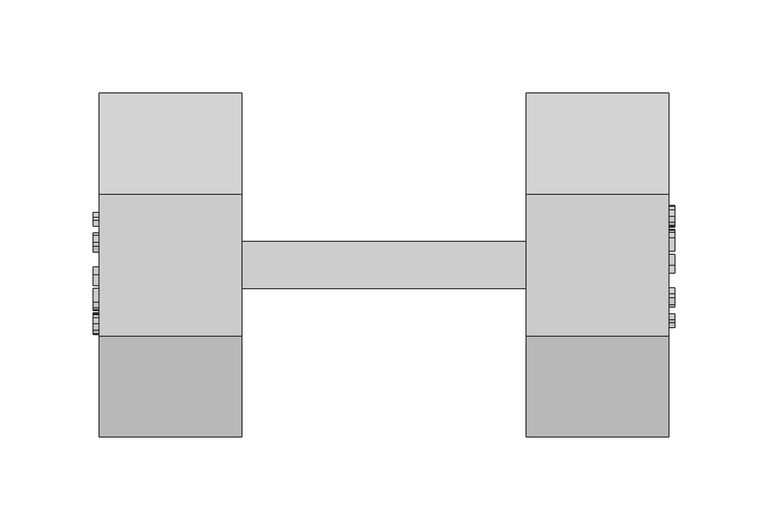
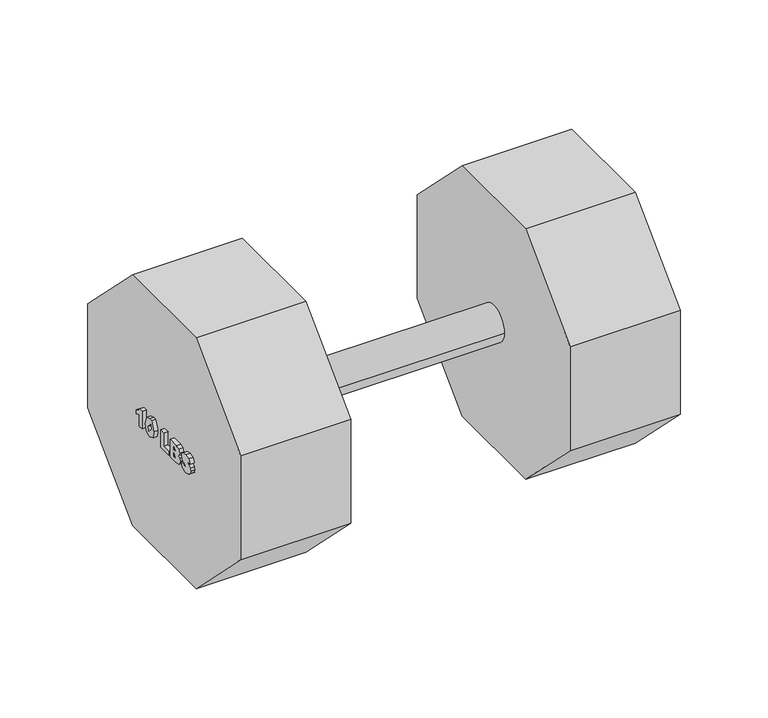
"""IFC4 building model written with IfcOpenShell, lengths in millimetres: proxy geometry."""

from ifc_helpers import new_model, si_unit, point, frame, frame_2d, origin, place, context, project, spatial, polyline, circle_curve, trimmed, segment, composite_curve, outline, extrude, source, transform, mapped, element, save


def generic_models_59bf1475(model_context):
    return source(origin(), model_context, "Body", "SweptSolid", [
        extrude(outline(polyline([(91.9815367, 53.8815367), (38.1, 0.0), (-38.1, 0.0), (-91.9815367, 53.8815367), (-91.9815367, 130.0815367), (-38.1, 183.9630735), (38.1, 183.9630735), (91.9815367, 130.0815367), (91.9815367, 53.8815367)])), frame((-76.2, 0.0, 0.0), z_axis=(1.0, 0.0, 0.0), x_axis=(0.0, 1.0, 0.0)), (0.0, 0.0, 1.0), 76.2),
        extrude(outline(composite_curve([segment(trimmed(circle_curve(frame_2d((0.0, 91.9815367)), 12.7), [point((12.7, 91.9815367))], [point((-12.7, 91.9815367))], False, "CARTESIAN"), True, "CONTINUOUS"), segment(trimmed(circle_curve(frame_2d((0.0, 91.9815367)), 12.7), [point((-12.7, 91.9815367))], [point((12.7, 91.9815367))], False, "CARTESIAN"), True, "CONTINUOUS")], self_intersect=False)), frame((0.0, 0.0, 0.0), z_axis=(1.0, 0.0, 0.0), x_axis=(0.0, 1.0, 0.0)), (0.0, 0.0, 1.0), 152.4),
        extrude(outline(polyline([(91.9815367, 53.8815367), (38.1, 0.0), (-38.1, 0.0), (-91.9815367, 53.8815367), (-91.9815367, 130.0815367), (-38.1, 183.9630735), (38.1, 183.9630735), (91.9815367, 130.0815367), (91.9815367, 53.8815367)])), frame((152.4, 0.0, 0.0), z_axis=(1.0, 0.0, 0.0), x_axis=(0.0, 1.0, 0.0)), (0.0, 0.0, 1.0), 76.2),
        extrude(outline(polyline([(20.9176471, 95.3120931), (23.7696998, 95.3120931), (25.3338542, 93.4016458), (28.1392157, 92.0748382), (28.1392157, 89.0866029), (26.0925858, 89.8920257), (24.4039216, 90.9931592), (24.4039216, 82.3630735), (20.9176471, 82.3630735), (20.9176471, 95.3120931)])), frame((-79.375, 0.0, 0.0), z_axis=(1.0, 0.0, 0.0), x_axis=(0.0, 1.0, 0.0)), (0.0, 0.0, 1.0), 3.175),
        extrude(outline(polyline([(17.1823529, 88.7636556), (16.9313879, 86.0614037), (16.2290748, 84.1334472), (14.6337929, 82.6276568), (12.0852328, 82.1140538), (8.1223192, 83.7248994), (6.972549, 88.8103467), (9.921875, 94.9949822), (11.9918505, 95.3120931), (15.9002911, 93.8588302), (17.1823529, 88.7636556)]), holes=[polyline([(13.6960784, 88.7247462), (10.8712623, 91.9678375), (10.4588235, 88.6313639), (13.2836397, 85.4758186), (13.6960784, 88.7247462)])]), frame((-79.375, 0.0, 0.0), z_axis=(1.0, 0.0, 0.0), x_axis=(0.0, 1.0, 0.0)), (0.0, 0.0, 1.0), 3.175),
        extrude(outline(polyline([(-0.9960784, 95.0630735), (-0.9960784, 82.3630735), (-10.9568627, 82.3630735), (-10.9568627, 85.3513087), (-4.9803922, 85.3513087), (-4.9803922, 95.0630735), (-0.9960784, 95.0630735)])), frame((-79.375, 0.0, 0.0), z_axis=(1.0, 0.0, 0.0), x_axis=(0.0, 1.0, 0.0)), (0.0, 0.0, 1.0), 3.175),
        extrude(outline(polyline([(-12.7, 95.0630735), (-12.7, 82.3630735), (-19.4546569, 82.3630735), (-22.6919118, 82.9506041), (-23.9467371, 84.1918112), (-24.4039216, 85.958294), (-23.7619179, 87.9660146), (-21.7619792, 89.0904938), (-23.1782782, 89.9426078), (-23.9058824, 91.8841825), (-22.9175858, 94.1487046), (-20.0849877, 95.0630735), (-12.7, 95.0630735)]), holes=[polyline([(-16.6843137, 85.3513087), (-16.6843137, 87.5924852), (-18.6258885, 85.3513087), (-16.6843137, 85.3513087)]), polyline([(-16.6843137, 90.0826813), (-16.6843137, 92.0748382), (-18.3379596, 90.0826813), (-16.6843137, 90.0826813)])]), frame((-79.375, 0.0, 0.0), z_axis=(1.0, 0.0, 0.0), x_axis=(0.0, 1.0, 0.0)), (0.0, 0.0, 1.0), 3.175),
        extrude(outline(polyline([(-25.6490196, 86.6041886), (-27.0536458, 83.3824975), (-31.5126532, 82.1140538), (-34.5553615, 82.6548933), (-36.4327359, 84.2443388), (-37.1039216, 86.530261), (-36.6019914, 88.4426537), (-34.9950368, 89.872571), (-32.6215686, 91.3277793), (-36.6058824, 91.5573443), (-35.1098192, 94.4132879), (-31.4581801, 95.3120931), (-28.3843444, 94.8140538), (-26.7054075, 93.4483369), (-26.1470588, 91.6040355), (-27.2481924, 89.1566396), (-30.897886, 87.6002671), (-31.5865809, 84.6042499), (-29.6333333, 86.8454264), (-25.6490196, 86.6041886)])), frame((-79.375, 0.0, 0.0), z_axis=(1.0, 0.0, 0.0), x_axis=(0.0, 1.0, 0.0)), (0.0, 0.0, 1.0), 3.175),
        extrude(outline(polyline([(-26.2557919, 99.036487), (-26.2557919, 86.0874674), (-29.7420665, 86.0874674), (-29.7420665, 94.7175531), (-31.4307307, 93.6164196), (-33.4773606, 92.8109968), (-33.4773606, 95.7992321), (-30.6719991, 97.1260397), (-29.1078446, 99.036487), (-26.2557919, 99.036487)])), frame((228.6, 0.0, 0.0), z_axis=(1.0, 0.0, 0.0), x_axis=(0.0, 1.0, 0.0)), (0.0, 0.0, 1.0), 3.175),
        extrude(outline(polyline([(-22.5204978, 92.4880495), (-21.2384359, 97.5832241), (-17.3299954, 99.036487), (-15.2600199, 98.7193761), (-12.3106939, 92.5347406), (-13.4604641, 87.4492933), (-17.4233777, 85.8384478), (-19.9719378, 86.3520507), (-21.5672196, 87.8578411), (-22.2695328, 89.7857976), (-22.5204978, 92.4880495)]), holes=[polyline([(-19.0342233, 92.4491402), (-18.6217846, 89.2002125), (-15.7969684, 92.3557578), (-16.2094071, 95.6922315), (-19.0342233, 92.4491402)])]), frame((228.6, 0.0, 0.0), z_axis=(1.0, 0.0, 0.0), x_axis=(0.0, 1.0, 0.0)), (0.0, 0.0, 1.0), 3.175),
        extrude(outline(polyline([(-4.3420665, 98.7874674), (-0.3577527, 98.7874674), (-0.3577527, 89.0757027), (5.6187179, 89.0757027), (5.6187179, 86.0874674), (-4.3420665, 86.0874674), (-4.3420665, 98.7874674)])), frame((228.6, 0.0, 0.0), z_axis=(1.0, 0.0, 0.0), x_axis=(0.0, 1.0, 0.0)), (0.0, 0.0, 1.0), 3.175),
        extrude(outline(polyline([(7.3618551, 98.7874674), (14.7468429, 98.7874674), (17.5794409, 97.8730985), (18.5677375, 95.6085764), (17.8401333, 93.6670017), (16.4238343, 92.8148877), (18.423773, 91.6904085), (19.0657767, 89.682688), (18.6085922, 87.9162051), (17.3537669, 86.674998), (14.116512, 86.0874674), (7.3618551, 86.0874674), (7.3618551, 98.7874674)]), holes=[polyline([(11.3461688, 93.8070752), (12.9998147, 93.8070752), (11.3461688, 95.7992321), (11.3461688, 93.8070752)]), polyline([(11.3461688, 89.0757027), (13.2877436, 89.0757027), (11.3461688, 91.3168791), (11.3461688, 89.0757027)])]), frame((228.6, 0.0, 0.0), z_axis=(1.0, 0.0, 0.0), x_axis=(0.0, 1.0, 0.0)), (0.0, 0.0, 1.0), 3.175),
        extrude(outline(polyline([(20.3108747, 90.3285826), (24.2951884, 90.5698203), (26.248436, 88.3286438), (25.5597411, 91.324661), (21.9100475, 92.8810335), (20.8089139, 95.3284294), (21.3672626, 97.1727308), (23.0461995, 98.5384478), (26.1200353, 99.036487), (29.7716744, 98.1376818), (31.2677375, 95.2817382), (27.2834237, 95.0521732), (29.6568919, 93.5969649), (31.2638465, 92.1670476), (31.7657767, 90.2546549), (31.094591, 87.9687327), (29.2172166, 86.3792872), (26.1745083, 85.8384478), (21.7155009, 87.1068914), (20.3108747, 90.3285826)])), frame((228.6, 0.0, 0.0), z_axis=(1.0, 0.0, 0.0), x_axis=(0.0, 1.0, 0.0)), (0.0, 0.0, 1.0), 3.175),
    ])


if __name__ == "__main__":
    model = new_model("IFC4")
    model_context = context("Model", 3, world=origin())
    ifc_project = project(units=[si_unit("LENGTHUNIT", "METRE", prefix="MILLI")], contexts=[model_context])
    site = spatial("IfcSite", under=ifc_project)
    building = spatial("IfcBuilding", under=site)
    placement = place(None, origin())
    generic_models_shape = generic_models_59bf1475(model_context)
    element("IfcBuildingElementProxy", 1, Name="Generic Models", at=placement, inside=building, context=model_context, shape_type="MappedRepresentation", body=[
        mapped(generic_models_shape, transform((0.0, 0.0, 0.0), x_axis=(1.0, 0.0, 0.0), y_axis=(0.0, 1.0, 0.0), z_axis=(0.0, 0.0, 1.0))),
    ])
    save(model, "model.ifc")

# Revit data of these elements
# Type
#   Text Depth = 0' - 0 1/8"
#   Text Color = none
#   Dumbell Material = none
#   Default Elevation = 0
